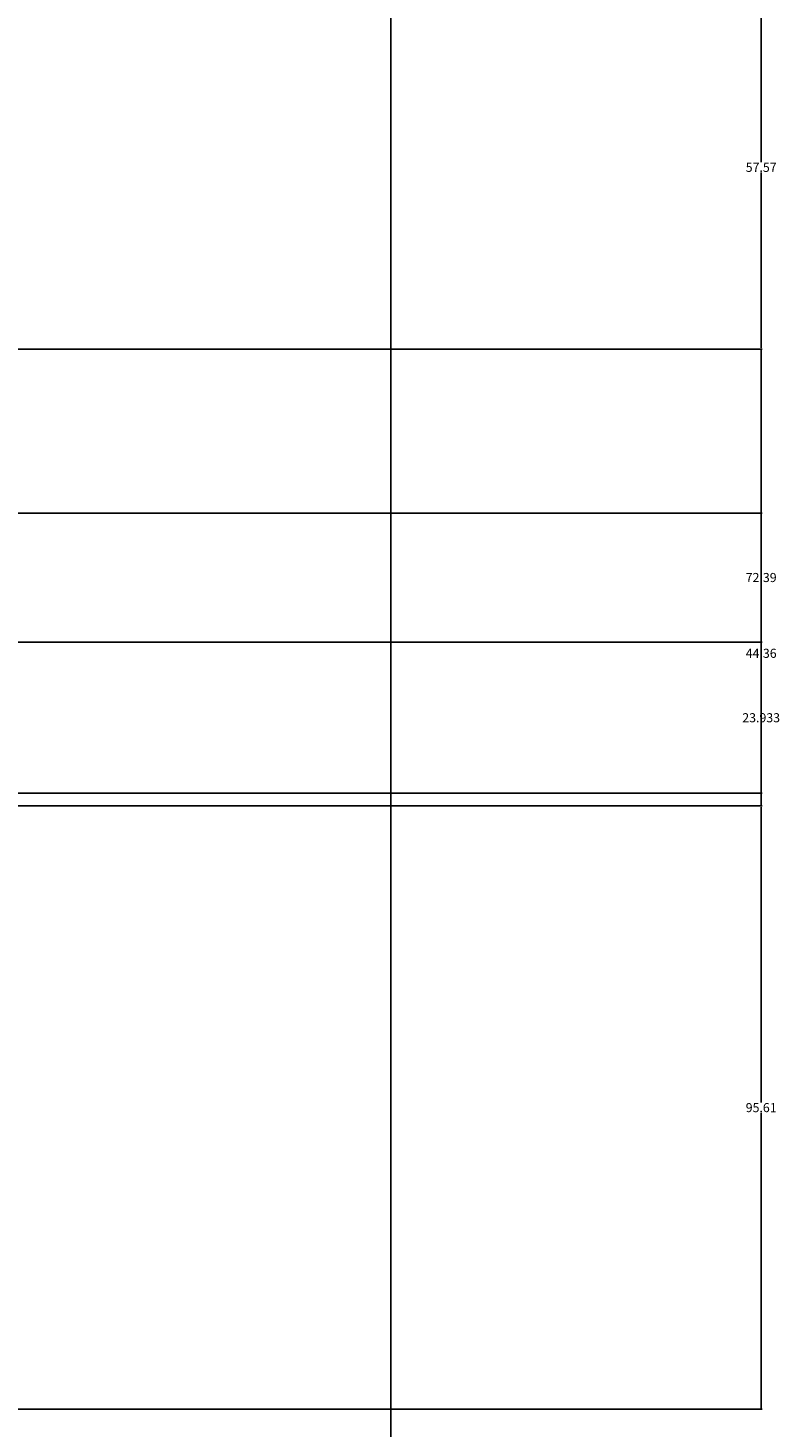
# Model space of a CAD drawing. Units: inches. Extents: x 241 to 943, y 109 to 1396.
# Tile 14 of 34: x 824 to 943, y 398 to 620. Entities that reach past the tile are written whole.
import ezdxf

# ---------------------------------------------------------------- set-up
doc = ezdxf.new("R2010")
doc.units = ezdxf.units.IN
doc.header["$MEASUREMENT"] = 0
doc.layers.add('A-ANNO-DIMS', color=2, linetype='Continuous', lineweight=18)
doc.styles.get("Standard").update_dxf_attribs({"font": 'arial.ttf'})
doc.dimstyles.get("Standard").update_dxf_attribs({"dimtxt": 1.4375, "dimasz": 0.18, "dimexe": 0.18, "dimexo": 0.0625, "dimgap": 0.09, "dimtad": 0, "dimtih": 1, "dimtoh": 1, "dimdec": 4, "dimzin": 0, "dimdsep": 46, "dimlunit": 4, "dimtxsty": 'Standard', "dimcen": 0.09, "dimadec": 0, "dimazin": 0, "dimtfac": 1, "dimtdec": 4, "dimtofl": 0, "dimtmove": 0, "dimatfit": 3, "dimfxl": 1, "dimtolj": 1, "dimtzin": 0, "dimarcsym": 0})

# ---------------------------------------------------------------- blocks, each defined once
blk = doc.blocks.new('*D6')
at = {"layer": 'A-ANNO-DIMS', "color": 0, "lineweight": -2, "transparency": 16777216}
for p, q in [((820.84, 232.89), (820.84, 1395.05)), ((821.02, 1394.87), (848.73, 1394.87)), ((881.49, 1394.87), (853.77, 1394.87)), ((881.67, 232.89), (881.67, 1395.05))]:
    blk.add_line(p, q, dxfattribs=at)
at = {"layer": 'A-ANNO-DIMS', "color": 0, "transparency": 16777216}
for points in [[(821.02, 1394.9), (821.02, 1394.84), (820.84, 1394.87)], [(881.49, 1394.9), (881.49, 1394.84), (881.67, 1394.87)]]:
    blk.add_solid(points, dxfattribs=at)
at = {"layer": 'Defpoints', "color": 0, "transparency": 16777216}
for p in [(881.67, 1394.87), (820.84, 232.83), (881.67, 232.83)]:
    blk.add_point(p, dxfattribs=at)
at = {"layer": 'A-ANNO-DIMS', "color": 0, "transparency": 16777216, "insert": (851.25, 1394.87), "char_height": 1.438, "attachment_point": 5}
blk.add_mtext('\\A1;60.83', dxfattribs=at)
blk = doc.blocks.new('*D31')
at = {"layer": 'A-ANNO-DIMS', "color": 0, "lineweight": -2, "transparency": 16777216}
for p, q in [((792.75, 496.44), (940.6, 496.44)), ((940.42, 496.26), (940.42, 449.46)), ((940.42, 401.01), (940.42, 447.81)), ((820.9, 400.83), (940.6, 400.83))]:
    blk.add_line(p, q, dxfattribs=at)
at = {"layer": 'A-ANNO-DIMS', "color": 0, "transparency": 16777216}
for points in [[(940.39, 496.26), (940.45, 496.26), (940.42, 496.44)], [(940.39, 401.01), (940.45, 401.01), (940.42, 400.83)]]:
    blk.add_solid(points, dxfattribs=at)
at = {"layer": 'Defpoints', "color": 0, "transparency": 16777216}
for p in [(792.69, 496.44), (940.42, 496.44), (820.84, 400.83)]:
    blk.add_point(p, dxfattribs=at)
at = {"layer": 'A-ANNO-DIMS', "color": 0, "transparency": 16777216, "insert": (940.42, 448.63), "char_height": 1.438, "attachment_point": 5}
blk.add_mtext('\\A1;95.61', dxfattribs=at)
blk = doc.blocks.new('*D45')
at = {"layer": 'A-ANNO-DIMS', "color": 0, "lineweight": -2, "transparency": 16777216}
for p, q in [((792.75, 568.83), (940.6, 568.83)), ((940.42, 568.65), (940.42, 533.46)), ((940.42, 496.62), (940.42, 531.81)), ((792.75, 496.44), (940.6, 496.44))]:
    blk.add_line(p, q, dxfattribs=at)
at = {"layer": 'A-ANNO-DIMS', "color": 0, "transparency": 16777216}
for points in [[(940.39, 568.65), (940.45, 568.65), (940.42, 568.83)], [(940.39, 496.62), (940.45, 496.62), (940.42, 496.44)]]:
    blk.add_solid(points, dxfattribs=at)
at = {"layer": 'Defpoints', "color": 0, "transparency": 16777216}
for p in [(792.69, 568.83), (940.42, 568.83), (792.69, 496.44)]:
    blk.add_point(p, dxfattribs=at)
at = {"layer": 'A-ANNO-DIMS', "color": 0, "transparency": 16777216, "insert": (940.42, 532.63), "char_height": 1.438, "attachment_point": 5}
blk.add_mtext('\\A1;72.39', dxfattribs=at)
blk = doc.blocks.new('*D85')
at = {"layer": 'A-ANNO-DIMS', "color": 0, "lineweight": -2, "transparency": 16777216}
for p, q in [((749.7, 626.4), (940.6, 626.4)), ((940.42, 626.22), (940.42, 598.44)), ((940.42, 569.01), (940.42, 596.79)), ((792.75, 568.83), (940.6, 568.83))]:
    blk.add_line(p, q, dxfattribs=at)
at = {"layer": 'A-ANNO-DIMS', "color": 0, "transparency": 16777216}
for points in [[(940.39, 626.22), (940.45, 626.22), (940.42, 626.4)], [(940.39, 569.01), (940.45, 569.01), (940.42, 568.83)]]:
    blk.add_solid(points, dxfattribs=at)
at = {"layer": 'Defpoints', "color": 0, "transparency": 16777216}
for p in [(749.63, 626.4), (940.42, 626.4), (792.69, 568.83)]:
    blk.add_point(p, dxfattribs=at)
at = {"layer": 'A-ANNO-DIMS', "color": 0, "transparency": 16777216, "insert": (940.42, 597.62), "char_height": 1.438, "attachment_point": 5}
blk.add_mtext('\\A1;57.57', dxfattribs=at)
blk = doc.blocks.new('*D145')
at = {"layer": 'A-ANNO-DIMS', "color": 0, "lineweight": -2, "transparency": 16777216}
for p, q in [((691.86, 522.37), (940.6, 522.37)), ((940.42, 522.19), (940.42, 511.23)), ((940.42, 498.62), (940.42, 509.58)), ((691.86, 498.44), (940.6, 498.44))]:
    blk.add_line(p, q, dxfattribs=at)
at = {"layer": 'A-ANNO-DIMS', "color": 0, "transparency": 16777216}
for points in [[(940.39, 522.19), (940.45, 522.19), (940.42, 522.37)], [(940.39, 498.62), (940.45, 498.62), (940.42, 498.44)]]:
    blk.add_solid(points, dxfattribs=at)
at = {"layer": 'Defpoints', "color": 0, "transparency": 16777216}
for p in [(691.79, 522.37), (940.42, 522.37), (691.79, 498.44)]:
    blk.add_point(p, dxfattribs=at)
at = {"layer": 'A-ANNO-DIMS', "color": 0, "transparency": 16777216, "insert": (940.42, 510.41), "char_height": 1.438, "attachment_point": 5}
blk.add_mtext('\\A1;23.933', dxfattribs=at)
blk = doc.blocks.new('*D146')
at = {"layer": 'A-ANNO-DIMS', "color": 0, "lineweight": -2, "transparency": 16777216}
for p, q in [((790.75, 542.8), (940.6, 542.8)), ((940.42, 542.62), (940.42, 521.44)), ((940.42, 498.62), (940.42, 519.8)), ((790.75, 498.44), (940.6, 498.44))]:
    blk.add_line(p, q, dxfattribs=at)
at = {"layer": 'A-ANNO-DIMS', "color": 0, "transparency": 16777216}
for points in [[(940.39, 542.62), (940.45, 542.62), (940.42, 542.8)], [(940.39, 498.62), (940.45, 498.62), (940.42, 498.44)]]:
    blk.add_solid(points, dxfattribs=at)
at = {"layer": 'Defpoints', "color": 0, "transparency": 16777216}
for p in [(790.69, 542.8), (940.42, 542.8), (790.69, 498.44)]:
    blk.add_point(p, dxfattribs=at)
at = {"layer": 'A-ANNO-DIMS', "color": 0, "transparency": 16777216, "insert": (940.42, 520.62), "char_height": 1.438, "attachment_point": 5}
blk.add_mtext('\\A1;44.36', dxfattribs=at)

msp = doc.modelspace()

# ---------------------------------------------------------------- dimensions: what is measured, and where the dimension line sits
at = {"layer": 'A-ANNO-DIMS'}
dim = msp.add_linear_dim(base=(881.667, 1394.8654), p1=(820.8374, 232.8295), p2=(881.667, 232.8295), dimstyle='Standard', override={"dimdec": 2, "dimlfac": 1, "dimrnd": 0, "dimzin": 0, "dimdsep": 46, "dimlunit": 2}, dxfattribs=at)
dim.commit()
dim.dimension.update_dxf_attribs({"geometry": '*D6', "text_midpoint": (851.2522, 1394.8654)})
for base, p1, p2, override, picture, middle in [((940.417, 626.4013), (792.691, 568.8295), (749.6328, 626.4013), {"dimdec": 2, "dimlfac": 1, "dimrnd": 0, "dimzin": 0, "dimdsep": 46, "dimlunit": 2}, '*D85', (940.417, 597.6154)), ((940.417, 568.8295), (792.691, 496.4395), (792.691, 568.8295), {"dimdec": 2, "dimlfac": 1, "dimrnd": 0, "dimzin": 0, "dimdsep": 46, "dimlunit": 2}, '*D45', (940.417, 532.6345)), ((940.417, 542.7994), (790.691, 498.4395), (790.691, 542.7994), {"dimdec": 2, "dimlfac": 1, "dimrnd": 0, "dimzin": 0, "dimdsep": 46, "dimlunit": 2}, '*D146', (940.417, 520.6194)), ((940.417, 522.3723), (691.794, 498.4395), (691.794, 522.3723), {"dimdec": 3, "dimlfac": 1, "dimrnd": 0, "dimzin": 0, "dimdsep": 46, "dimlunit": 2}, '*D145', (940.417, 510.4059)), ((940.417, 496.4395), (820.8374, 400.8295), (792.691, 496.4395), {"dimdec": 2, "dimlfac": 1, "dimrnd": 0, "dimzin": 0, "dimdsep": 46, "dimlunit": 2}, '*D31', (940.417, 448.6345))]:
    dim = msp.add_linear_dim(base=base, p1=p1, p2=p2, angle=90, dimstyle='Standard', override=override, dxfattribs=at)
    dim.commit()
    dim.dimension.update_dxf_attribs({"geometry": picture, "text_midpoint": middle})

doc.saveas('drawing.dxf')
